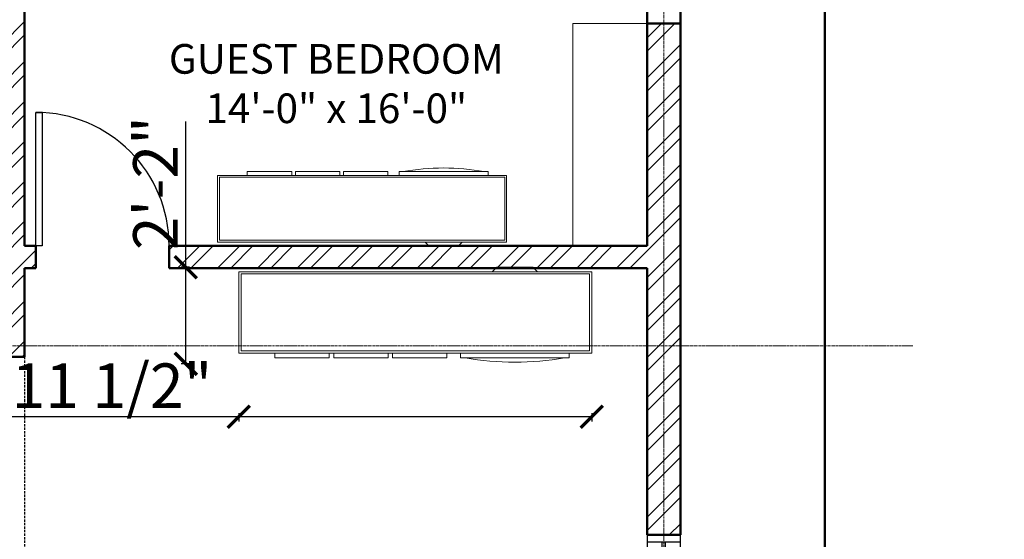
# Model space of a CAD drawing. Units: inches. Extents: x 261 to 2725, y 291 to 1454.
# Tile 14 of 35: x 777 to 1043, y 951 to 1091. Entities that reach past the tile are written whole.
import ezdxf

# ---------------------------------------------------------------- set-up
doc = ezdxf.new("R2010")
doc.units = ezdxf.units.IN
doc.linetypes.add('CENTER', pattern=[2, 1.25, -0.25, 0.25, -0.25])
doc.linetypes.add('DASHED', pattern=[19.05, 12.7, -6.35])
for name, color, linetype, lineweight in [('A-ANNO-DIMS', 136, 'Continuous', 18), ('A-AREA-IDEN', 18, 'Continuous', 18), ('A-DOOR', 160, 'Continuous', 25), ('A-FLOR-FIXT', 145, 'Continuous', 18), ('A-FURN', 30, 'Continuous', 18), ('A-GLAZ', 150, 'Continuous', 25), ('A-GRID', 251, 'CENTER', 13), ('A-WALL', 222, 'Continuous', 50), ('A-WALL-OVHD', 222, 'DASHED', 25), ('A-WALL-PATT', 243, 'Continuous', 13)]:
    doc.layers.add(name, color=color, linetype=linetype, lineweight=lineweight)
doc.styles.get("Standard").update_dxf_attribs({"font": 'arial.ttf'})
doc.dimstyles.new('ISO-25', dxfattribs={"dimtxt": 12, "dimasz": 6, "dimexe": 1.25, "dimexo": 0.625, "dimtad": 1, "dimdec": 0, "dimlunit": 3, "dimtxsty": 'Standard', "dimblk": 'ARCHTICK', "dimcen": 2.5, "dimadec": 0, "dimazin": 0, "dimtfac": 1, "dimtdec": 0, "dimtmove": 0, "dimatfit": 3, "dimfxl": 1, "dimfxlon": 1, "dimarcsym": 0})

# ---------------------------------------------------------------- blocks, each defined once
blk = doc.blocks.new('*U12')
for p, q in [((0, 0), (0, -6)), ((36, 0), (36, -6))]:
    blk.add_line(p, q)
blk.add_lwpolyline([(0, 0), (0, 36), (1.75, 36), (1.75, 0)], close=True)
blk.add_arc((0, 0), 36, 0, 90)
blk = doc.blocks.new('Entertainment Center')
for p, q in [((-4, 0), (-5, -1)), ((4, 0), (-4, 0)), ((5, -1), (4, 0)), ((-17, -19), (-17, -1)), ((-17, -1), (61, -1)), ((-16.5, -18.5), (-16.5, -1.5)), ((-16.5, -1.5), (60.5, -1.5)), ((60.5, -1.5), (60.5, -18.5)), ((61, -1), (61, -19)), ((61, -19), (-17, -19)), ((60.5, -18.5), (-16.5, -18.5)), ((-12, -20), (-12, -19)), ((12, -19), (12, -20)), ((15, -20), (15, -19)), ((27, -19), (27, -20)), ((28, -20), (28, -19)), ((40, -19), (40, -20)), ((41, -20), (41, -19)), ((53, -19), (53, -20)), ((12, -20), (-12, -20)), ((27, -20), (15, -20)), ((40, -20), (28, -20)), ((53, -20), (41, -20))]:
    blk.add_line(p, q)
blk.add_arc((0, 40), 61, 259.6111, 280.3889)
blk = doc.blocks.new('WIN-72')
for p, q in [((955.45, 950.47), (946.45, 950.47)), ((950.45, 950.47), (950.45, 882.47)), ((951.45, 882.47), (951.45, 950.47)), ((946.45, 882.47), (955.45, 882.47))]:
    blk.add_line(p, q)
blk.add_lwpolyline([(955.45, 880.47), (955.45, 952.47), (946.45, 952.47), (946.45, 880.47)], close=True)
blk = doc.blocks.new('_ArchTick')
at = {"color": 0, "linetype": 'ByBlock', "const_width": 0.15}
blk.add_lwpolyline([(-0.5, -0.5), (0.5, 0.5)], dxfattribs=at)
blk = doc.blocks.new('*D47')
at = {"layer": 'A-ANNO-DIMS', "color": 0, "lineweight": -2, "ltscale": 0.07, "transparency": 16777216}
for p, q in [((836.24, 984.34), (689.66, 984.34)), ((836.24, 985.34), (836.24, 983.09)), ((931.53, 984.34), (836.24, 984.34)), ((931.53, 985.34), (931.53, 983.09))]:
    blk.add_line(p, q, dxfattribs=at)
at = {"layer": 'Defpoints', "color": 0, "ltscale": 0.07, "transparency": 16777216}
for p in [(836.24, 998.63), (931.53, 998.63), (836.24, 984.34)]:
    blk.add_point(p, dxfattribs=at)
at = {"layer": 'A-ANNO-DIMS', "color": 0, "lineweight": -2, "ltscale": 0.07, "transparency": 16777216, "xscale": 6, "yscale": 6, "zscale": 6, "rotation": 180}
blk.add_blockref('_ArchTick', (836.24, 984.34), dxfattribs=at)
at = {"layer": 'A-ANNO-DIMS', "color": 0, "lineweight": -2, "ltscale": 0.07, "transparency": 16777216, "xscale": 6, "yscale": 6, "zscale": 6}
blk.add_blockref('_ArchTick', (931.53, 984.34), dxfattribs=at)
at = {"layer": 'A-ANNO-DIMS', "color": 0, "ltscale": 0.07, "transparency": 16777216, "insert": (759.95, 991.17), "char_height": 12, "attachment_point": 5}
blk.add_mtext('TV UNIT 7\'-11 1/2"', dxfattribs=at)
blk = doc.blocks.new('*D48')
at = {"layer": 'A-ANNO-DIMS', "color": 0, "lineweight": -2, "ltscale": 0.07, "transparency": 16777216}
for p, q in [((821.95, 1024.69), (821.95, 1064.04)), ((822.95, 1024.69), (820.7, 1024.69)), ((821.95, 998.63), (821.95, 1024.69)), ((822.95, 998.63), (820.7, 998.63))]:
    blk.add_line(p, q, dxfattribs=at)
at = {"layer": 'Defpoints', "color": 0, "ltscale": 0.07, "transparency": 16777216}
for p in [(821.95, 1024.69), (836.24, 1024.69), (836.24, 998.63)]:
    blk.add_point(p, dxfattribs=at)
at = {"layer": 'A-ANNO-DIMS', "color": 0, "lineweight": -2, "ltscale": 0.07, "transparency": 16777216, "xscale": 6, "yscale": 6, "zscale": 6}
for p, rotation in [((821.95, 1024.69), 90), ((821.95, 998.63), 270)]:
    blk.add_blockref('_ArchTick', p, dxfattribs=dict(at, rotation=rotation))
at = {"layer": 'A-ANNO-DIMS', "color": 0, "ltscale": 0.07, "transparency": 16777216, "insert": (815.3, 1047.37), "char_height": 12, "attachment_point": 5, "rotation": 90}
blk.add_mtext('2\'-2"', dxfattribs=at)
blk = doc.blocks.new('*D84')
at = {"layer": 'A-ANNO-DIMS', "color": 0, "lineweight": -2, "ltscale": 0.07, "transparency": 16777216}
for p, q in [((2600.96, 1024.47), (2603.21, 1024.47)), ((2601.96, 799.47), (2601.96, 1024.47)), ((2600.96, 799.47), (2603.21, 799.47))]:
    blk.add_line(p, q, dxfattribs=at)
at = {"layer": 'Defpoints', "color": 0, "ltscale": 0.07, "transparency": 16777216}
for p in [(946.45, 1024.47), (2601.96, 1024.47), (946.45, 799.47)]:
    blk.add_point(p, dxfattribs=at)
at = {"layer": 'A-ANNO-DIMS', "color": 0, "lineweight": -2, "ltscale": 0.07, "transparency": 16777216, "xscale": 6, "yscale": 6, "zscale": 6}
for p, rotation in [((2601.96, 1024.47), 90), ((2601.96, 799.47), 270)]:
    blk.add_blockref('_ArchTick', p, dxfattribs=dict(at, rotation=rotation))
at = {"layer": 'A-ANNO-DIMS', "color": 0, "ltscale": 0.07, "transparency": 16777216, "insert": (2595.21, 911.97), "char_height": 12, "attachment_point": 5, "rotation": 90}
blk.add_mtext('18\'-9"', dxfattribs=at)
blk = doc.blocks.new('*D85')
at = {"layer": 'A-ANNO-DIMS', "color": 0, "lineweight": -2, "ltscale": 0.07, "transparency": 16777216}
for p, q in [((2600.96, 1222.47), (2603.21, 1222.47)), ((2601.96, 1024.47), (2601.96, 1222.47)), ((2600.96, 1024.47), (2603.21, 1024.47))]:
    blk.add_line(p, q, dxfattribs=at)
at = {"layer": 'Defpoints', "color": 0, "ltscale": 0.07, "transparency": 16777216}
for p in [(946.45, 1222.47), (2601.96, 1222.47), (946.45, 1024.47)]:
    blk.add_point(p, dxfattribs=at)
at = {"layer": 'A-ANNO-DIMS', "color": 0, "lineweight": -2, "ltscale": 0.07, "transparency": 16777216, "xscale": 6, "yscale": 6, "zscale": 6}
for p, rotation in [((2601.96, 1222.47), 90), ((2601.96, 1024.47), 270)]:
    blk.add_blockref('_ArchTick', p, dxfattribs=dict(at, rotation=rotation))
at = {"layer": 'A-ANNO-DIMS', "color": 0, "ltscale": 0.07, "transparency": 16777216, "insert": (2595.21, 1123.47), "char_height": 12, "attachment_point": 5, "rotation": 90}
blk.add_mtext('16\'-6"', dxfattribs=at)
blk = doc.blocks.new('*D103')
at = {"layer": 'A-ANNO-DIMS', "color": 0, "lineweight": -2, "ltscale": 0.07, "transparency": 16777216}
for p, q in [((287.06, 1231.47), (284.81, 1231.47)), ((286.06, 439.47), (286.06, 1231.47)), ((287.06, 439.47), (284.81, 439.47))]:
    blk.add_line(p, q, dxfattribs=at)
at = {"layer": 'Defpoints', "color": 0, "ltscale": 0.07, "transparency": 16777216}
for p in [(286.06, 1231.47), (1243.08, 1231.47), (1243.08, 439.47)]:
    blk.add_point(p, dxfattribs=at)
at = {"layer": 'A-ANNO-DIMS', "color": 0, "lineweight": -2, "ltscale": 0.07, "transparency": 16777216, "xscale": 6, "yscale": 6, "zscale": 6}
for p, rotation in [((286.06, 1231.47), 90), ((286.06, 439.47), 270)]:
    blk.add_blockref('_ArchTick', p, dxfattribs=dict(at, rotation=rotation))
at = {"layer": 'A-ANNO-DIMS', "color": 0, "ltscale": 0.07, "transparency": 16777216, "insert": (279.3, 835.47), "char_height": 12, "attachment_point": 5, "rotation": 90}
blk.add_mtext('66\'-0"', dxfattribs=at)
blk = doc.blocks.new('*D109')
at = {"layer": 'A-ANNO-DIMS', "color": 0, "lineweight": -2, "ltscale": 0.07, "transparency": 16777216}
for p, q in [((287.06, 964.47), (284.81, 964.47)), ((286.06, 799.47), (286.06, 964.47)), ((287.06, 799.47), (284.81, 799.47))]:
    blk.add_line(p, q, dxfattribs=at)
at = {"layer": 'Defpoints', "color": 0, "ltscale": 0.07, "transparency": 16777216}
for p in [(286.06, 964.47), (1252.08, 964.47), (1252.08, 799.47)]:
    blk.add_point(p, dxfattribs=at)
at = {"layer": 'A-ANNO-DIMS', "color": 0, "lineweight": -2, "ltscale": 0.07, "transparency": 16777216, "xscale": 6, "yscale": 6, "zscale": 6}
for p, rotation in [((286.06, 964.47), 90), ((286.06, 799.47), 270)]:
    blk.add_blockref('_ArchTick', p, dxfattribs=dict(at, rotation=rotation))
at = {"layer": 'A-ANNO-DIMS', "color": 0, "ltscale": 0.07, "transparency": 16777216, "insert": (279.3, 881.97), "char_height": 12, "attachment_point": 5, "rotation": 90}
blk.add_mtext('13\'-9"', dxfattribs=at)
blk = doc.blocks.new('*D110')
at = {"layer": 'A-ANNO-DIMS', "color": 0, "lineweight": -2, "ltscale": 0.07, "transparency": 16777216}
for p, q in [((287.06, 1222.47), (284.81, 1222.47)), ((286.06, 964.47), (286.06, 1222.47)), ((287.06, 964.47), (284.81, 964.47))]:
    blk.add_line(p, q, dxfattribs=at)
at = {"layer": 'Defpoints', "color": 0, "ltscale": 0.07, "transparency": 16777216}
for p in [(286.06, 1222.47), (1252.08, 1222.47), (1252.08, 964.47)]:
    blk.add_point(p, dxfattribs=at)
at = {"layer": 'A-ANNO-DIMS', "color": 0, "lineweight": -2, "ltscale": 0.07, "transparency": 16777216, "xscale": 6, "yscale": 6, "zscale": 6}
for p, rotation in [((286.06, 1222.47), 90), ((286.06, 964.47), 270)]:
    blk.add_blockref('_ArchTick', p, dxfattribs=dict(at, rotation=rotation))
at = {"layer": 'A-ANNO-DIMS', "color": 0, "ltscale": 0.07, "transparency": 16777216, "insert": (279.3, 1093.47), "char_height": 12, "attachment_point": 5, "rotation": 90}
blk.add_mtext('21\'-6"', dxfattribs=at)
blk = doc.blocks.new('*D123')
at = {"layer": 'A-ANNO-DIMS', "color": 0, "lineweight": -2, "ltscale": 0.07, "transparency": 16777216}
for p, q in [((287.06, 1054.85), (284.81, 1054.85)), ((286.06, 439.47), (286.06, 1054.85)), ((287.06, 439.47), (284.81, 439.47))]:
    blk.add_line(p, q, dxfattribs=at)
at = {"layer": 'Defpoints', "color": 0, "ltscale": 0.07, "transparency": 16777216}
for p in [(286.06, 1054.85), (2007.71, 1054.85), (2007.71, 439.47)]:
    blk.add_point(p, dxfattribs=at)
at = {"layer": 'A-ANNO-DIMS', "color": 0, "lineweight": -2, "ltscale": 0.07, "transparency": 16777216, "xscale": 6, "yscale": 6, "zscale": 6}
for p, rotation in [((286.06, 1054.85), 90), ((286.06, 439.47), 270)]:
    blk.add_blockref('_ArchTick', p, dxfattribs=dict(at, rotation=rotation))
at = {"layer": 'A-ANNO-DIMS', "color": 0, "ltscale": 0.07, "transparency": 16777216, "insert": (279.22, 747.16), "char_height": 12, "attachment_point": 5, "rotation": 90}
blk.add_mtext('51\'-3 1/2"', dxfattribs=at)

msp = doc.modelspace()

# ---------------------------------------------------------------- hatches: boundary and pattern name
at = {"layer": 'A-WALL-PATT'}
h = msp.add_hatch(dxfattribs=at)
h.set_pattern_fill('ANSI32', color=256, scale=0.8)
h.paths.add_polyline_path([(478.45, 685.47), (580.45, 685.47), (580.45, 691.47), (577.45, 691.47), (577.45, 694.47), (571.45, 694.47), (571.45, 691.47), (478.45, 691.47), (478.45, 721.47), (469.45, 721.47), (469.45, 508.47), (538.45, 508.47), (538.45, 517.47), (478.45, 517.47)])
h.paths.add_polyline_path([(694.45, 517.47), (676.45, 517.47), (676.45, 646.47), (670.45, 646.47), (670.45, 517.47), (610.45, 517.47), (610.45, 508.47), (694.45, 508.47)])
h.paths.add_polyline_path([(676.45, 784.47), (478.45, 784.47), (478.45, 844.47), (469.45, 844.47), (469.45, 745.47), (478.45, 745.47), (478.45, 775.47), (571.45, 775.47), (571.45, 724.47), (577.45, 724.47), (577.45, 775.47), (670.45, 775.47), (670.45, 691.47), (610.45, 691.47), (610.45, 685.47), (670.45, 685.47), (670.45, 682.47), (676.45, 682.47)])
h.paths.add_polyline_path([(955.45, 880.47), (946.45, 880.47), (946.45, 808.47), (778.45, 808.47), (778.45, 799.47), (946.45, 799.47), (946.45, 517.47), (898.45, 517.47), (898.45, 508.47), (955.45, 508.47)])
h.paths.add_polyline_path([(778.45, 598.47), (772.45, 598.47), (772.45, 517.47), (754.45, 517.47), (754.45, 508.47), (826.45, 508.47), (826.45, 517.47), (778.45, 517.47)])
h.paths.add_polyline_path([(955.45, 1090.47), (946.45, 1090.47), (946.45, 1030.47), (817.45, 1030.47), (817.45, 1024.47), (946.45, 1024.47), (946.45, 952.47), (955.45, 952.47)])
h.paths.add_polyline_path([(955.45, 1231.47), (730.45, 1231.47), (730.45, 1222.47), (772.45, 1222.47), (772.45, 1096.47), (766.45, 1096.47), (766.45, 1090.47), (772.45, 1090.47), (772.45, 1006.47), (712.45, 1006.47), (712.45, 1000.47), (778.45, 1000.47), (778.45, 1024.47), (781.45, 1024.47), (781.45, 1030.47), (778.45, 1030.47), (778.45, 1222.47), (946.45, 1222.47), (946.45, 1162.47), (955.45, 1162.47)])
h.paths.add_polyline_path([(694.45, 1231.47), (619.45, 1231.47), (619.45, 1222.47), (646.45, 1222.47), (646.45, 1039.47), (652.45, 1039.47), (652.45, 1090.47), (736.45, 1090.47), (736.45, 1096.47), (652.45, 1096.47), (652.45, 1222.47), (694.45, 1222.47)])
h.paths.add_polyline_path([(571.45, 1231.47), (469.45, 1231.47), (469.45, 1099.47), (478.45, 1099.47), (478.45, 1144.47), (544.45, 1144.47), (544.45, 1153.47), (538.45, 1153.47), (538.45, 1150.47), (478.45, 1150.47), (478.45, 1222.47), (538.45, 1222.47), (538.45, 1183.47), (544.45, 1183.47), (544.45, 1222.47), (571.45, 1222.47)])
h.paths.add_polyline_path([(538.45, 1006.47), (478.45, 1006.47), (478.45, 1051.47), (469.45, 1051.47), (469.45, 940.47), (478.45, 940.47), (478.45, 1000.47), (538.45, 1000.47)])
h.paths.add_polyline_path([(652.45, 1006.47), (652.45, 1009.47), (646.45, 1009.47), (646.45, 1006.47), (586.45, 1006.47), (586.45, 1000.47), (652.45, 1000.47)])
h.paths.add_polyline_path([(1288.08, 973.47), (1243.08, 973.47), (1243.08, 920.97), (1252.08, 920.97), (1252.08, 964.47), (1288.08, 964.47)], flags=17)
h.paths.add_polyline_path([(1402.08, 805.47), (1252.08, 805.47), (1252.08, 848.97), (1243.08, 848.97), (1243.08, 757.47), (1252.08, 757.47), (1252.08, 799.47), (1294.08, 799.47), (1372.08, 799.47), (1372.08, 779.47), (1372.08, 715.47), (1378.08, 715.47), (1378.08, 799.47), (1402.08, 799.47)])
h.paths.add_polyline_path([(1252.08, 721.47), (1243.08, 721.47), (1243.08, 439.47), (1729.08, 439.47), (1729.08, 709.47), (1720.08, 709.47), (1720.08, 679.47), (1582.08, 679.47), (1582.08, 670.47), (1588.08, 670.47), (1588.08, 673.47), (1720.08, 673.47), (1720.08, 559.47), (1690.08, 559.47), (1690.08, 550.47), (1720.08, 550.47), (1720.08, 448.47), (1252.08, 448.47), (1252.08, 496.47), (1312.08, 496.47), (1312.08, 505.47), (1252.08, 505.47), (1252.08, 673.47), (1405.08, 673.47), (1405.08, 679.47), (1378.08, 679.47), (1378.08, 685.47), (1372.08, 685.47), (1372.08, 679.47), (1252.08, 679.47)])
h.paths.add_polyline_path([(1450.08, 550.47), (1480.08, 550.47), (1480.08, 559.47), (1450.08, 559.47), (1450.08, 679.47), (1441.08, 679.47), (1441.08, 673.47), (1444.08, 673.47), (1444.08, 505.47), (1384.08, 505.47), (1384.08, 496.47), (1450.08, 496.47)], flags=17)
h.paths.add_polyline_path([(1618.08, 559.47), (1588.08, 559.47), (1588.08, 634.47), (1582.08, 634.47), (1582.08, 559.47), (1552.08, 559.47), (1552.08, 550.47), (1618.08, 550.47)], flags=17)
h.paths.add_polyline_path([(1564.08, 964.47), (1630.08, 964.47), (1630.08, 973.47), (1477.08, 973.47), (1477.08, 964.47), (1558.08, 964.47), (1558.08, 926.22), (1558.08, 887.97), (1486.08, 887.97), (1486.08, 881.97), (1558.08, 881.97), (1558.08, 805.47), (1450.08, 805.47), (1450.08, 845.97), (1444.08, 845.97), (1444.08, 805.47), (1438.08, 805.47), (1438.08, 799.47), (1564.08, 799.47)], flags=17)
h.paths.add_polyline_path([(1453.08, 973.47), (1408.08, 973.47), (1408.08, 964.47), (1444.08, 964.47), (1444.08, 881.97), (1450.08, 881.97), (1456.08, 881.97), (1456.08, 887.97), (1450.08, 887.97), (1450.08, 964.47), (1453.08, 964.47)], flags=17)
h.paths.add_polyline_path([(1729.08, 1231.47), (1243.08, 1231.47), (1243.08, 1167.47), (1252.08, 1167.47), (1252.08, 1222.47), (1441.08, 1222.47), (1441.08, 1045.47), (1648.08, 1045.47), (1648.08, 1051.47), (1450.08, 1051.47), (1450.08, 1074.47), (1450.08, 1222.47), (1472.08, 1222.47), (1720.08, 1222.47), (1720.08, 1051.47), (1708.08, 1051.47), (1708.08, 1045.47), (1720.08, 1045.47), (1720.08, 973.47), (1702.08, 973.47), (1702.08, 964.47), (1720.08, 964.47), (1720.08, 769.47), (1729.08, 769.47)])
h.paths.add_polyline_path([(2493.71, 1054.85), (2007.71, 1054.85), (2007.71, 439.47), (2214.67, 439.47), (2214.67, 496.47), (2493.71, 496.47)])
h.paths.add_polyline_path([(2016.71, 1045.85), (2304.71, 1045.85), (2304.71, 841.47), (2310.71, 841.47), (2310.71, 1045.85), (2484.71, 1045.85), (2484.71, 805.47), (2310.71, 805.47), (2310.71, 811.47), (2304.71, 811.47), (2304.71, 799.47), (2484.71, 799.47), (2484.71, 679.47), (2304.71, 679.47), (2304.71, 673.47), (2484.71, 673.47), (2484.71, 505.47), (2208.67, 505.47), (2208.67, 448.47), (2016.71, 448.47), (2016.71, 799.47), (2304.71, 799.47), (2304.71, 805.47), (2016.71, 805.47)], flags=16)

# ---------------------------------------------------------------- linework, layer by layer
at = {"layer": 'A-FURN'}
for q in [(926.45, 1030.47), (946.45, 1090.47)]:
    msp.add_line((926.45, 1090.47), q, dxfattribs=at)
at = {"layer": 'A-GRID', "ltscale": 0.5}
for p, q in [((950.95, 1330.47), (950.95, 416.47)), ((394.31, 1003.47), (1018.31, 1003.47))]:
    msp.add_line(p, q, dxfattribs=at)
at = {"layer": 'A-WALL'}
for p, q in [((994.45, 1270.47), (994.45, 412.47)), ((778.45, 1222.47), (778.45, 1030.47)), ((946.45, 1090.47), (955.45, 1090.47)), ((946.45, 1090.47), (946.45, 1030.47)), ((955.45, 1090.47), (955.45, 952.47)), ((778.45, 1030.47), (781.45, 1030.47)), ((781.45, 1030.47), (781.45, 1024.47)), ((817.45, 1030.47), (817.45, 1024.47)), ((817.45, 1030.47), (946.45, 1030.47)), ((778.45, 1024.47), (781.45, 1024.47)), ((778.45, 1024.47), (778.45, 1000.47)), ((817.45, 1024.47), (946.45, 1024.47)), ((946.45, 1024.47), (946.45, 952.47)), ((778.45, 1000.47), (712.45, 1000.47)), ((946.45, 952.47), (955.45, 952.47))]:
    msp.add_line(p, q, dxfattribs=at)
msp.add_lwpolyline([(955.45, 1090.47), (955.45, 1162.47), (946.45, 1162.47), (946.45, 1090.47)], close=True, dxfattribs=at)
at = {"layer": 'A-WALL-OVHD', "ltscale": 0.05}
msp.add_line((778.45, 1000.47), (778.45, 799.47), dxfattribs=at)

# ---------------------------------------------------------------- block references
at = {"layer": 'A-DOOR'}
msp.add_blockref('*U12', (781.45, 1030.47), dxfattribs=at)
at = {"layer": 'A-FLOR-FIXT', "rotation": 180}
msp.add_blockref('Entertainment Center', (891.53, 1030.47), dxfattribs=at)
at = {"layer": 'A-FLOR-FIXT', "xscale": -1.221586140170944, "yscale": 1.221586140170944, "zscale": 1.221586140170944}
msp.add_blockref('Entertainment Center', (910.76, 1024.69), dxfattribs=at)
at = {"layer": 'A-GLAZ'}
msp.add_blockref('WIN-72', (0, 0), dxfattribs=at)

# ---------------------------------------------------------------- texts
at = {"layer": 'A-AREA-IDEN', "insert": (810.82, 1084.9), "char_height": 8, "attachment_point": 1}
msp.add_mtext_dynamic_manual_height_columns('\\pxqc;{\\fTimes New Roman|b0|i0|c0|p18;GUEST BEDROOM\\P14\'-0" x 16\'-0"}', width=103.5273, gutter_width=12.5, heights=[0], dxfattribs=at)

# ---------------------------------------------------------------- dimensions: what is measured, and where the dimension line sits
at = {"layer": 'A-ANNO-DIMS', "ltscale": 0.07}
for base, p1, p2, override, picture, middle in [((286.06, 1231.47), (1243.08, 439.47), (1243.08, 1231.47), {"dimdec": 1, "dimlfac": 1, "dimrnd": 0, "dimzin": 1, "dimdsep": 46, "dimlunit": 4, "dimfrac": 2}, '*D103', (279.3, 835.47)), ((286.06, 1222.47), (1252.08, 964.47), (1252.08, 1222.47), {"dimdec": 1, "dimlfac": 1, "dimrnd": 0, "dimzin": 1, "dimdsep": 46, "dimlunit": 4, "dimfrac": 2}, '*D110', (279.3, 1093.47)), ((2601.96, 1222.47), (946.45, 1024.47), (946.45, 1222.47), {"dimdec": 1, "dimlfac": 1, "dimrnd": 0, "dimzin": 1, "dimdsep": 46, "dimlunit": 4, "dimfrac": 2}, '*D85', (2595.21, 1123.47)), ((821.95, 1024.69), (836.24, 998.63), (836.24, 1024.69), {"dimdec": 1, "dimrnd": 0, "dimzin": 1, "dimlunit": 4, "dimfrac": 2}, '*D48', (815.3, 1047.37)), ((286.06, 1054.85), (2007.71, 439.47), (2007.71, 1054.85), {"dimdec": 1, "dimlfac": 1, "dimrnd": 0, "dimzin": 1, "dimdsep": 46, "dimlunit": 4, "dimfrac": 2}, '*D123', (279.22, 747.16)), ((2601.96, 1024.47), (946.45, 799.47), (946.45, 1024.47), {"dimdec": 1, "dimlfac": 1, "dimrnd": 0, "dimzin": 1, "dimdsep": 46, "dimlunit": 4, "dimfrac": 2}, '*D84', (2595.21, 911.97)), ((286.06, 964.47), (1252.08, 799.47), (1252.08, 964.47), {"dimdec": 1, "dimlfac": 1, "dimrnd": 0, "dimzin": 1, "dimdsep": 46, "dimlunit": 4, "dimfrac": 2}, '*D109', (279.3, 881.97))]:
    dim = msp.add_linear_dim(base=base, p1=p1, p2=p2, angle=90, dimstyle='ISO-25', override=override, dxfattribs=at)
    dim.commit()
    dim.dimension.update_dxf_attribs({"geometry": picture, "text_midpoint": middle})
dim = msp.add_linear_dim(base=(836.24, 984.34), p1=(931.53, 998.63), p2=(836.24, 998.63), angle=180, text='TV UNIT <>', dimstyle='ISO-25', override={"dimdec": 1, "dimrnd": 0, "dimzin": 1, "dimlunit": 4, "dimfrac": 2}, dxfattribs=at)
dim.commit()
dim.dimension.update_dxf_attribs({"geometry": '*D47', "text_midpoint": (759.95, 991.17)})

doc.saveas('drawing.dxf')
